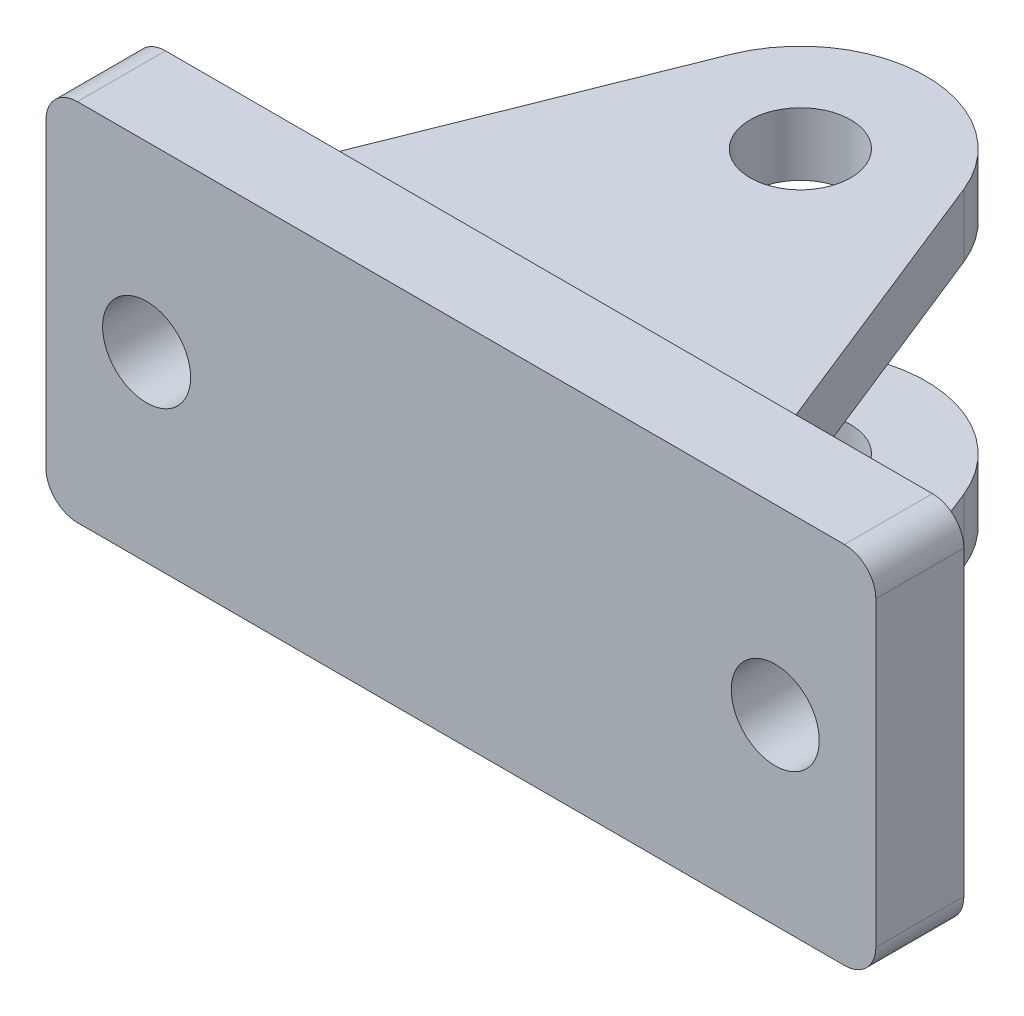
ISO-10303-21;
HEADER;
FILE_DESCRIPTION(('STEP AP214'),'2;1');
FILE_NAME('part.step','',(''),(''),'','','');
FILE_SCHEMA(('AUTOMOTIVE_DESIGN { 1 0 10303 214 1 1 1 1 }'));
ENDSEC;
DATA;
#1=APPLICATION_CONTEXT('core data for automotive mechanical design processes');
#2=APPLICATION_PROTOCOL_DEFINITION('international standard','automotive_design',2000,#1);
#3=PRODUCT_CONTEXT('',#1,'mechanical');
#4=PRODUCT('Part','Part','',(#3));
#5=PRODUCT_RELATED_PRODUCT_CATEGORY('part','',(#4));
#6=PRODUCT_DEFINITION_FORMATION('','',#4);
#7=PRODUCT_DEFINITION_CONTEXT('part definition',#1,'design');
#8=PRODUCT_DEFINITION('design','',#6,#7);
#9=PRODUCT_DEFINITION_SHAPE('','',#8);
#10=(LENGTH_UNIT() NAMED_UNIT(*) SI_UNIT(.MILLI.,.METRE.));
#11=(NAMED_UNIT(*) PLANE_ANGLE_UNIT() SI_UNIT($,.RADIAN.));
#12=(NAMED_UNIT(*) SI_UNIT($,.STERADIAN.) SOLID_ANGLE_UNIT());
#13=UNCERTAINTY_MEASURE_WITH_UNIT(LENGTH_MEASURE(1.E-05),#10,'distance_accuracy_value','');
#14=(GEOMETRIC_REPRESENTATION_CONTEXT(3) GLOBAL_UNCERTAINTY_ASSIGNED_CONTEXT((#13)) GLOBAL_UNIT_ASSIGNED_CONTEXT((#10,
#11,#12)) REPRESENTATION_CONTEXT('',''));
#15=CARTESIAN_POINT('',(0.,0.,0.));
#16=DIRECTION('',(0.,0.,1.));
#17=DIRECTION('',(1.,0.,0.));
#18=AXIS2_PLACEMENT_3D('',#15,#16,#17);
#19=CARTESIAN_POINT('',(-61.,24.,0.));
#20=DIRECTION('',(0.,0.,-1.));
#21=DIRECTION('',(-1.,0.,0.));
#22=AXIS2_PLACEMENT_3D('',#19,#20,#21);
#23=PLANE('',#22);
#24=DIRECTION('',(1.,0.,0.));
#25=VECTOR('',#24,1.);
#26=CARTESIAN_POINT('',(-37.5,-26.,0.));
#27=LINE('',#26,#25);
#28=CARTESIAN_POINT('',(-37.5,-26.,0.));
#29=VERTEX_POINT('',#28);
#30=CARTESIAN_POINT('',(37.5,-26.,0.));
#31=VERTEX_POINT('',#30);
#32=EDGE_CURVE('E176',#29,#31,#27,.T.);
#33=ORIENTED_EDGE('',*,*,#32,.T.);
#34=DIRECTION('',(0.,1.,0.));
#35=VECTOR('',#34,1.);
#36=CARTESIAN_POINT('',(37.5,-26.,0.));
#37=LINE('',#36,#35);
#38=CARTESIAN_POINT('',(37.5,-16.,0.));
#39=VERTEX_POINT('',#38);
#40=EDGE_CURVE('E163',#31,#39,#37,.T.);
#41=ORIENTED_EDGE('',*,*,#40,.T.);
#42=DIRECTION('',(1.,0.,0.));
#43=VECTOR('',#42,1.);
#44=CARTESIAN_POINT('',(-37.5,-16.,0.));
#45=LINE('',#44,#43);
#46=CARTESIAN_POINT('',(-37.5,-16.,0.));
#47=VERTEX_POINT('',#46);
#48=EDGE_CURVE('E189',#47,#39,#45,.T.);
#49=ORIENTED_EDGE('',*,*,#48,.F.);
#50=DIRECTION('',(0.,1.,0.));
#51=VECTOR('',#50,1.);
#52=CARTESIAN_POINT('',(-37.5,-26.,0.));
#53=LINE('',#52,#51);
#54=EDGE_CURVE('E191',#29,#47,#53,.T.);
#55=ORIENTED_EDGE('',*,*,#54,.F.);
#56=EDGE_LOOP('',(#33,#41,#49,#55));
#57=FACE_BOUND('',#56,.T.);
#58=CARTESIAN_POINT('',(-50.,0.,0.));
#59=DIRECTION('',(0.,0.,1.));
#60=DIRECTION('',(1.,0.,0.));
#61=AXIS2_PLACEMENT_3D('',#58,#59,#60);
#62=CIRCLE('',#61,7.);
#63=CARTESIAN_POINT('',(-43.,0.,0.));
#64=VERTEX_POINT('',#63);
#65=EDGE_CURVE('E235',#64,#64,#62,.T.);
#66=ORIENTED_EDGE('',*,*,#65,.T.);
#67=EDGE_LOOP('',(#66));
#68=FACE_BOUND('',#67,.T.);
#69=CARTESIAN_POINT('',(-61.,24.,0.));
#70=DIRECTION('',(0.,0.,1.));
#71=DIRECTION('',(-1.,0.,0.));
#72=AXIS2_PLACEMENT_3D('',#69,#70,#71);
#73=CIRCLE('',#72,5.);
#74=CARTESIAN_POINT('',(-61.,29.,0.));
#75=VERTEX_POINT('',#74);
#76=CARTESIAN_POINT('',(-66.,24.,0.));
#77=VERTEX_POINT('',#76);
#78=EDGE_CURVE('E236',#75,#77,#73,.T.);
#79=ORIENTED_EDGE('',*,*,#78,.F.);
#80=DIRECTION('',(-1.,0.,0.));
#81=VECTOR('',#80,1.);
#82=CARTESIAN_POINT('',(-61.,29.,0.));
#83=LINE('',#82,#81);
#84=CARTESIAN_POINT('',(61.,29.,0.));
#85=VERTEX_POINT('',#84);
#86=EDGE_CURVE('E241',#85,#75,#83,.T.);
#87=ORIENTED_EDGE('',*,*,#86,.F.);
#88=CARTESIAN_POINT('',(61.,24.,0.));
#89=DIRECTION('',(0.,0.,1.));
#90=DIRECTION('',(-1.,0.,0.));
#91=AXIS2_PLACEMENT_3D('',#88,#89,#90);
#92=CIRCLE('',#91,5.);
#93=CARTESIAN_POINT('',(66.,24.,0.));
#94=VERTEX_POINT('',#93);
#95=EDGE_CURVE('E275',#94,#85,#92,.T.);
#96=ORIENTED_EDGE('',*,*,#95,.F.);
#97=DIRECTION('',(0.,1.,0.));
#98=VECTOR('',#97,1.);
#99=CARTESIAN_POINT('',(66.,24.,0.));
#100=LINE('',#99,#98);
#101=CARTESIAN_POINT('',(66.,-24.,0.));
#102=VERTEX_POINT('',#101);
#103=EDGE_CURVE('E269',#102,#94,#100,.T.);
#104=ORIENTED_EDGE('',*,*,#103,.F.);
#105=CARTESIAN_POINT('',(61.,-24.,0.));
#106=DIRECTION('',(0.,0.,1.));
#107=DIRECTION('',(1.,0.,0.));
#108=AXIS2_PLACEMENT_3D('',#105,#106,#107);
#109=CIRCLE('',#108,5.);
#110=CARTESIAN_POINT('',(61.,-29.,0.));
#111=VERTEX_POINT('',#110);
#112=EDGE_CURVE('E268',#111,#102,#109,.T.);
#113=ORIENTED_EDGE('',*,*,#112,.F.);
#114=DIRECTION('',(1.,0.,0.));
#115=VECTOR('',#114,1.);
#116=CARTESIAN_POINT('',(-61.,-29.,0.));
#117=LINE('',#116,#115);
#118=CARTESIAN_POINT('',(-61.,-29.,0.));
#119=VERTEX_POINT('',#118);
#120=EDGE_CURVE('E266',#119,#111,#117,.T.);
#121=ORIENTED_EDGE('',*,*,#120,.F.);
#122=CARTESIAN_POINT('',(-61.,-24.,0.));
#123=DIRECTION('',(0.,0.,1.));
#124=DIRECTION('',(-1.,0.,0.));
#125=AXIS2_PLACEMENT_3D('',#122,#123,#124);
#126=CIRCLE('',#125,5.);
#127=CARTESIAN_POINT('',(-66.,-24.,0.));
#128=VERTEX_POINT('',#127);
#129=EDGE_CURVE('E262',#128,#119,#126,.T.);
#130=ORIENTED_EDGE('',*,*,#129,.F.);
#131=DIRECTION('',(0.,-1.,0.));
#132=VECTOR('',#131,1.);
#133=CARTESIAN_POINT('',(-66.,24.,0.));
#134=LINE('',#133,#132);
#135=EDGE_CURVE('E265',#77,#128,#134,.T.);
#136=ORIENTED_EDGE('',*,*,#135,.F.);
#137=EDGE_LOOP('',(#79,#87,#96,#104,#113,#121,#130,#136));
#138=FACE_BOUND('',#137,.T.);
#139=CARTESIAN_POINT('',(50.,0.,0.));
#140=DIRECTION('',(0.,0.,1.));
#141=DIRECTION('',(-1.,0.,0.));
#142=AXIS2_PLACEMENT_3D('',#139,#140,#141);
#143=CIRCLE('',#142,7.);
#144=CARTESIAN_POINT('',(43.,0.,0.));
#145=VERTEX_POINT('',#144);
#146=EDGE_CURVE('E227',#145,#145,#143,.T.);
#147=ORIENTED_EDGE('',*,*,#146,.T.);
#148=EDGE_LOOP('',(#147));
#149=FACE_BOUND('',#148,.T.);
#150=DIRECTION('',(1.,0.,0.));
#151=VECTOR('',#150,1.);
#152=CARTESIAN_POINT('',(-37.5,26.,0.));
#153=LINE('',#152,#151);
#154=CARTESIAN_POINT('',(-37.5,26.,0.));
#155=VERTEX_POINT('',#154);
#156=CARTESIAN_POINT('',(37.5,26.,0.));
#157=VERTEX_POINT('',#156);
#158=EDGE_CURVE('E206',#155,#157,#153,.T.);
#159=ORIENTED_EDGE('',*,*,#158,.F.);
#160=DIRECTION('',(0.,-1.,0.));
#161=VECTOR('',#160,1.);
#162=CARTESIAN_POINT('',(-37.5,26.,0.));
#163=LINE('',#162,#161);
#164=CARTESIAN_POINT('',(-37.5,16.,0.));
#165=VERTEX_POINT('',#164);
#166=EDGE_CURVE('E225',#155,#165,#163,.T.);
#167=ORIENTED_EDGE('',*,*,#166,.T.);
#168=DIRECTION('',(1.,0.,0.));
#169=VECTOR('',#168,1.);
#170=CARTESIAN_POINT('',(-37.5,16.,0.));
#171=LINE('',#170,#169);
#172=CARTESIAN_POINT('',(37.5,16.,0.));
#173=VERTEX_POINT('',#172);
#174=EDGE_CURVE('E212',#165,#173,#171,.T.);
#175=ORIENTED_EDGE('',*,*,#174,.T.);
#176=DIRECTION('',(0.,-1.,0.));
#177=VECTOR('',#176,1.);
#178=CARTESIAN_POINT('',(37.5,26.,0.));
#179=LINE('',#178,#177);
#180=EDGE_CURVE('E219',#157,#173,#179,.T.);
#181=ORIENTED_EDGE('',*,*,#180,.F.);
#182=EDGE_LOOP('',(#159,#167,#175,#181));
#183=FACE_BOUND('',#182,.T.);
#184=ADVANCED_FACE('F39',(#57,#68,#138,#149,#183),#23,.T.);
#185=CARTESIAN_POINT('',(-61.,24.,14.));
#186=DIRECTION('',(0.,0.,-1.));
#187=DIRECTION('',(-1.,0.,0.));
#188=AXIS2_PLACEMENT_3D('',#185,#186,#187);
#189=PLANE('',#188);
#190=CARTESIAN_POINT('',(-61.,24.,14.));
#191=DIRECTION('',(0.,0.,1.));
#192=DIRECTION('',(-1.,0.,0.));
#193=AXIS2_PLACEMENT_3D('',#190,#191,#192);
#194=CIRCLE('',#193,5.);
#195=CARTESIAN_POINT('',(-61.,29.,14.));
#196=VERTEX_POINT('',#195);
#197=CARTESIAN_POINT('',(-66.,24.,14.));
#198=VERTEX_POINT('',#197);
#199=EDGE_CURVE('E243',#196,#198,#194,.T.);
#200=ORIENTED_EDGE('',*,*,#199,.T.);
#201=DIRECTION('',(0.,-1.,0.));
#202=VECTOR('',#201,1.);
#203=CARTESIAN_POINT('',(-66.,24.,14.));
#204=LINE('',#203,#202);
#205=CARTESIAN_POINT('',(-66.,-24.,14.));
#206=VERTEX_POINT('',#205);
#207=EDGE_CURVE('E245',#198,#206,#204,.T.);
#208=ORIENTED_EDGE('',*,*,#207,.T.);
#209=CARTESIAN_POINT('',(-61.,-24.,14.));
#210=DIRECTION('',(0.,0.,1.));
#211=DIRECTION('',(-1.,0.,0.));
#212=AXIS2_PLACEMENT_3D('',#209,#210,#211);
#213=CIRCLE('',#212,5.);
#214=CARTESIAN_POINT('',(-61.,-29.,14.));
#215=VERTEX_POINT('',#214);
#216=EDGE_CURVE('E250',#206,#215,#213,.T.);
#217=ORIENTED_EDGE('',*,*,#216,.T.);
#218=DIRECTION('',(1.,0.,0.));
#219=VECTOR('',#218,1.);
#220=CARTESIAN_POINT('',(-61.,-29.,14.));
#221=LINE('',#220,#219);
#222=CARTESIAN_POINT('',(61.,-29.,14.));
#223=VERTEX_POINT('',#222);
#224=EDGE_CURVE('E248',#215,#223,#221,.T.);
#225=ORIENTED_EDGE('',*,*,#224,.T.);
#226=CARTESIAN_POINT('',(61.,-24.,14.));
#227=DIRECTION('',(0.,0.,1.));
#228=DIRECTION('',(1.,0.,0.));
#229=AXIS2_PLACEMENT_3D('',#226,#227,#228);
#230=CIRCLE('',#229,5.);
#231=CARTESIAN_POINT('',(66.,-24.,14.));
#232=VERTEX_POINT('',#231);
#233=EDGE_CURVE('E253',#223,#232,#230,.T.);
#234=ORIENTED_EDGE('',*,*,#233,.T.);
#235=DIRECTION('',(0.,1.,0.));
#236=VECTOR('',#235,1.);
#237=CARTESIAN_POINT('',(66.,24.,14.));
#238=LINE('',#237,#236);
#239=CARTESIAN_POINT('',(66.,24.,14.));
#240=VERTEX_POINT('',#239);
#241=EDGE_CURVE('E251',#232,#240,#238,.T.);
#242=ORIENTED_EDGE('',*,*,#241,.T.);
#243=CARTESIAN_POINT('',(61.,24.,14.));
#244=DIRECTION('',(0.,0.,1.));
#245=DIRECTION('',(-1.,0.,0.));
#246=AXIS2_PLACEMENT_3D('',#243,#244,#245);
#247=CIRCLE('',#246,5.);
#248=CARTESIAN_POINT('',(61.,29.,14.));
#249=VERTEX_POINT('',#248);
#250=EDGE_CURVE('E254',#240,#249,#247,.T.);
#251=ORIENTED_EDGE('',*,*,#250,.T.);
#252=DIRECTION('',(-1.,0.,0.));
#253=VECTOR('',#252,1.);
#254=CARTESIAN_POINT('',(-61.,29.,14.));
#255=LINE('',#254,#253);
#256=EDGE_CURVE('E260',#249,#196,#255,.T.);
#257=ORIENTED_EDGE('',*,*,#256,.T.);
#258=EDGE_LOOP('',(#200,#208,#217,#225,#234,#242,#251,#257));
#259=FACE_BOUND('',#258,.T.);
#260=CARTESIAN_POINT('',(-50.,0.,14.));
#261=DIRECTION('',(0.,0.,1.));
#262=DIRECTION('',(1.,0.,0.));
#263=AXIS2_PLACEMENT_3D('',#260,#261,#262);
#264=CIRCLE('',#263,7.);
#265=CARTESIAN_POINT('',(-43.,0.,14.));
#266=VERTEX_POINT('',#265);
#267=EDGE_CURVE('E234',#266,#266,#264,.T.);
#268=ORIENTED_EDGE('',*,*,#267,.F.);
#269=EDGE_LOOP('',(#268));
#270=FACE_BOUND('',#269,.T.);
#271=CARTESIAN_POINT('',(50.,0.,14.));
#272=DIRECTION('',(0.,0.,1.));
#273=DIRECTION('',(-1.,0.,0.));
#274=AXIS2_PLACEMENT_3D('',#271,#272,#273);
#275=CIRCLE('',#274,7.);
#276=CARTESIAN_POINT('',(43.,0.,14.));
#277=VERTEX_POINT('',#276);
#278=EDGE_CURVE('E230',#277,#277,#275,.T.);
#279=ORIENTED_EDGE('',*,*,#278,.F.);
#280=EDGE_LOOP('',(#279));
#281=FACE_BOUND('',#280,.T.);
#282=ADVANCED_FACE('F312',(#259,#270,#281),#189,.F.);
#283=CARTESIAN_POINT('',(-61.,24.,14.));
#284=DIRECTION('',(0.,0.,-1.));
#285=DIRECTION('',(-1.,0.,0.));
#286=AXIS2_PLACEMENT_3D('',#283,#284,#285);
#287=CYLINDRICAL_SURFACE('',#286,5.);
#288=ORIENTED_EDGE('',*,*,#78,.T.);
#289=DIRECTION('',(0.,0.,-1.));
#290=VECTOR('',#289,1.);
#291=CARTESIAN_POINT('',(-66.,24.,14.));
#292=LINE('',#291,#290);
#293=EDGE_CURVE('E11',#198,#77,#292,.T.);
#294=ORIENTED_EDGE('',*,*,#293,.F.);
#295=ORIENTED_EDGE('',*,*,#199,.F.);
#296=DIRECTION('',(0.,0.,-1.));
#297=VECTOR('',#296,1.);
#298=CARTESIAN_POINT('',(-61.,29.,14.));
#299=LINE('',#298,#297);
#300=EDGE_CURVE('E259',#196,#75,#299,.T.);
#301=ORIENTED_EDGE('',*,*,#300,.T.);
#302=EDGE_LOOP('',(#288,#294,#295,#301));
#303=FACE_BOUND('',#302,.T.);
#304=ADVANCED_FACE('F41',(#303),#287,.T.);
#305=CARTESIAN_POINT('',(-66.,24.,14.));
#306=DIRECTION('',(1.,0.,0.));
#307=DIRECTION('',(0.,0.,-1.));
#308=AXIS2_PLACEMENT_3D('',#305,#306,#307);
#309=PLANE('',#308);
#310=ORIENTED_EDGE('',*,*,#135,.T.);
#311=DIRECTION('',(0.,0.,-1.));
#312=VECTOR('',#311,1.);
#313=CARTESIAN_POINT('',(-66.,-24.,14.));
#314=LINE('',#313,#312);
#315=EDGE_CURVE('E50',#206,#128,#314,.T.);
#316=ORIENTED_EDGE('',*,*,#315,.F.);
#317=ORIENTED_EDGE('',*,*,#207,.F.);
#318=ORIENTED_EDGE('',*,*,#293,.T.);
#319=EDGE_LOOP('',(#310,#316,#317,#318));
#320=FACE_BOUND('',#319,.T.);
#321=ADVANCED_FACE('F319',(#320),#309,.F.);
#322=CARTESIAN_POINT('',(-61.,-24.,14.));
#323=DIRECTION('',(0.,0.,-1.));
#324=DIRECTION('',(-1.,0.,0.));
#325=AXIS2_PLACEMENT_3D('',#322,#323,#324);
#326=CYLINDRICAL_SURFACE('',#325,5.);
#327=ORIENTED_EDGE('',*,*,#129,.T.);
#328=DIRECTION('',(0.,0.,-1.));
#329=VECTOR('',#328,1.);
#330=CARTESIAN_POINT('',(-61.,-29.,14.));
#331=LINE('',#330,#329);
#332=EDGE_CURVE('E288',#215,#119,#331,.T.);
#333=ORIENTED_EDGE('',*,*,#332,.F.);
#334=ORIENTED_EDGE('',*,*,#216,.F.);
#335=ORIENTED_EDGE('',*,*,#315,.T.);
#336=EDGE_LOOP('',(#327,#333,#334,#335));
#337=FACE_BOUND('',#336,.T.);
#338=ADVANCED_FACE('F298',(#337),#326,.T.);
#339=CARTESIAN_POINT('',(-61.,-29.,14.));
#340=DIRECTION('',(0.,1.,0.));
#341=DIRECTION('',(0.,0.,1.));
#342=AXIS2_PLACEMENT_3D('',#339,#340,#341);
#343=PLANE('',#342);
#344=ORIENTED_EDGE('',*,*,#120,.T.);
#345=DIRECTION('',(0.,0.,-1.));
#346=VECTOR('',#345,1.);
#347=CARTESIAN_POINT('',(61.,-29.,14.));
#348=LINE('',#347,#346);
#349=EDGE_CURVE('E286',#223,#111,#348,.T.);
#350=ORIENTED_EDGE('',*,*,#349,.F.);
#351=ORIENTED_EDGE('',*,*,#224,.F.);
#352=ORIENTED_EDGE('',*,*,#332,.T.);
#353=EDGE_LOOP('',(#344,#350,#351,#352));
#354=FACE_BOUND('',#353,.T.);
#355=ADVANCED_FACE('F307',(#354),#343,.F.);
#356=CARTESIAN_POINT('',(61.,-24.,14.));
#357=DIRECTION('',(0.,0.,-1.));
#358=DIRECTION('',(-1.,0.,0.));
#359=AXIS2_PLACEMENT_3D('',#356,#357,#358);
#360=CYLINDRICAL_SURFACE('',#359,5.);
#361=ORIENTED_EDGE('',*,*,#112,.T.);
#362=DIRECTION('',(0.,0.,-1.));
#363=VECTOR('',#362,1.);
#364=CARTESIAN_POINT('',(66.,-24.,14.));
#365=LINE('',#364,#363);
#366=EDGE_CURVE('E282',#232,#102,#365,.T.);
#367=ORIENTED_EDGE('',*,*,#366,.F.);
#368=ORIENTED_EDGE('',*,*,#233,.F.);
#369=ORIENTED_EDGE('',*,*,#349,.T.);
#370=EDGE_LOOP('',(#361,#367,#368,#369));
#371=FACE_BOUND('',#370,.T.);
#372=ADVANCED_FACE('F313',(#371),#360,.T.);
#373=CARTESIAN_POINT('',(66.,24.,14.));
#374=DIRECTION('',(-1.,0.,0.));
#375=DIRECTION('',(0.,-1.,0.));
#376=AXIS2_PLACEMENT_3D('',#373,#374,#375);
#377=PLANE('',#376);
#378=ORIENTED_EDGE('',*,*,#103,.T.);
#379=DIRECTION('',(0.,0.,-1.));
#380=VECTOR('',#379,1.);
#381=CARTESIAN_POINT('',(66.,24.,14.));
#382=LINE('',#381,#380);
#383=EDGE_CURVE('E278',#240,#94,#382,.T.);
#384=ORIENTED_EDGE('',*,*,#383,.F.);
#385=ORIENTED_EDGE('',*,*,#241,.F.);
#386=ORIENTED_EDGE('',*,*,#366,.T.);
#387=EDGE_LOOP('',(#378,#384,#385,#386));
#388=FACE_BOUND('',#387,.T.);
#389=ADVANCED_FACE('F334',(#388),#377,.F.);
#390=CARTESIAN_POINT('',(61.,24.,14.));
#391=DIRECTION('',(0.,0.,-1.));
#392=DIRECTION('',(-1.,0.,0.));
#393=AXIS2_PLACEMENT_3D('',#390,#391,#392);
#394=CYLINDRICAL_SURFACE('',#393,5.);
#395=ORIENTED_EDGE('',*,*,#95,.T.);
#396=DIRECTION('',(0.,0.,-1.));
#397=VECTOR('',#396,1.);
#398=CARTESIAN_POINT('',(61.,29.,14.));
#399=LINE('',#398,#397);
#400=EDGE_CURVE('E280',#249,#85,#399,.T.);
#401=ORIENTED_EDGE('',*,*,#400,.F.);
#402=ORIENTED_EDGE('',*,*,#250,.F.);
#403=ORIENTED_EDGE('',*,*,#383,.T.);
#404=EDGE_LOOP('',(#395,#401,#402,#403));
#405=FACE_BOUND('',#404,.T.);
#406=ADVANCED_FACE('F332',(#405),#394,.T.);
#407=CARTESIAN_POINT('',(-61.,29.,14.));
#408=DIRECTION('',(0.,-1.,0.));
#409=DIRECTION('',(0.,0.,-1.));
#410=AXIS2_PLACEMENT_3D('',#407,#408,#409);
#411=PLANE('',#410);
#412=ORIENTED_EDGE('',*,*,#86,.T.);
#413=ORIENTED_EDGE('',*,*,#300,.F.);
#414=ORIENTED_EDGE('',*,*,#256,.F.);
#415=ORIENTED_EDGE('',*,*,#400,.T.);
#416=EDGE_LOOP('',(#412,#413,#414,#415));
#417=FACE_BOUND('',#416,.T.);
#418=ADVANCED_FACE('F326',(#417),#411,.F.);
#419=CARTESIAN_POINT('',(-50.,0.,14.));
#420=DIRECTION('',(0.,0.,-1.));
#421=DIRECTION('',(-1.,0.,0.));
#422=AXIS2_PLACEMENT_3D('',#419,#420,#421);
#423=CYLINDRICAL_SURFACE('',#422,7.);
#424=ORIENTED_EDGE('',*,*,#267,.T.);
#425=EDGE_LOOP('',(#424));
#426=FACE_BOUND('',#425,.T.);
#427=ORIENTED_EDGE('',*,*,#65,.F.);
#428=EDGE_LOOP('',(#427));
#429=FACE_BOUND('',#428,.T.);
#430=ADVANCED_FACE('F351',(#426,#429),#423,.F.);
#431=CARTESIAN_POINT('',(50.,0.,14.));
#432=DIRECTION('',(0.,0.,-1.));
#433=DIRECTION('',(-1.,0.,0.));
#434=AXIS2_PLACEMENT_3D('',#431,#432,#433);
#435=CYLINDRICAL_SURFACE('',#434,7.);
#436=ORIENTED_EDGE('',*,*,#278,.T.);
#437=EDGE_LOOP('',(#436));
#438=FACE_BOUND('',#437,.T.);
#439=ORIENTED_EDGE('',*,*,#146,.F.);
#440=EDGE_LOOP('',(#439));
#441=FACE_BOUND('',#440,.T.);
#442=ADVANCED_FACE('F358',(#438,#441),#435,.F.);
#443=CARTESIAN_POINT('',(0.,26.,-40.));
#444=DIRECTION('',(0.,1.,0.));
#445=DIRECTION('',(0.,0.,1.));
#446=AXIS2_PLACEMENT_3D('',#443,#444,#445);
#447=PLANE('',#446);
#448=CARTESIAN_POINT('',(0.,26.,-40.));
#449=DIRECTION('',(0.,1.,0.));
#450=DIRECTION('',(0.,0.,1.));
#451=AXIS2_PLACEMENT_3D('',#448,#449,#450);
#452=CIRCLE('',#451,20.);
#453=CARTESIAN_POINT('',(18.5750206115008,26.,-47.414081823282));
#454=VERTEX_POINT('',#453);
#455=CARTESIAN_POINT('',(-18.5750206115008,26.,-47.414081823282));
#456=VERTEX_POINT('',#455);
#457=EDGE_CURVE('E199',#454,#456,#452,.T.);
#458=ORIENTED_EDGE('',*,*,#457,.T.);
#459=DIRECTION('',(-0.3707040911641,0.,0.92875103057504));
#460=VECTOR('',#459,1.);
#461=CARTESIAN_POINT('',(-37.5,26.,0.));
#462=LINE('',#461,#460);
#463=EDGE_CURVE('E201',#456,#155,#462,.T.);
#464=ORIENTED_EDGE('',*,*,#463,.T.);
#465=ORIENTED_EDGE('',*,*,#158,.T.);
#466=DIRECTION('',(-0.3707040911641,0.,-0.92875103057504));
#467=VECTOR('',#466,1.);
#468=CARTESIAN_POINT('',(37.5,26.,0.));
#469=LINE('',#468,#467);
#470=EDGE_CURVE('E64',#157,#454,#469,.T.);
#471=ORIENTED_EDGE('',*,*,#470,.T.);
#472=EDGE_LOOP('',(#458,#464,#465,#471));
#473=FACE_BOUND('',#472,.T.);
#474=CARTESIAN_POINT('',(0.,26.,-40.));
#475=DIRECTION('',(0.,1.,0.));
#476=DIRECTION('',(0.,0.,1.));
#477=AXIS2_PLACEMENT_3D('',#474,#475,#476);
#478=CIRCLE('',#477,8.);
#479=CARTESIAN_POINT('',(0.,26.,-32.));
#480=VERTEX_POINT('',#479);
#481=EDGE_CURVE('E193',#480,#480,#478,.T.);
#482=ORIENTED_EDGE('',*,*,#481,.F.);
#483=EDGE_LOOP('',(#482));
#484=FACE_BOUND('',#483,.T.);
#485=ADVANCED_FACE('F365',(#473,#484),#447,.T.);
#486=CARTESIAN_POINT('',(0.,16.,-40.));
#487=DIRECTION('',(0.,1.,0.));
#488=DIRECTION('',(0.,0.,1.));
#489=AXIS2_PLACEMENT_3D('',#486,#487,#488);
#490=PLANE('',#489);
#491=CARTESIAN_POINT('',(0.,16.,-40.));
#492=DIRECTION('',(0.,1.,0.));
#493=DIRECTION('',(0.,0.,1.));
#494=AXIS2_PLACEMENT_3D('',#491,#492,#493);
#495=CIRCLE('',#494,20.);
#496=CARTESIAN_POINT('',(18.5750206115008,16.,-47.414081823282));
#497=VERTEX_POINT('',#496);
#498=CARTESIAN_POINT('',(-18.5750206115008,16.,-47.414081823282));
#499=VERTEX_POINT('',#498);
#500=EDGE_CURVE('E197',#497,#499,#495,.T.);
#501=ORIENTED_EDGE('',*,*,#500,.F.);
#502=DIRECTION('',(-0.3707040911641,0.,-0.92875103057504));
#503=VECTOR('',#502,1.);
#504=CARTESIAN_POINT('',(37.5,16.,0.));
#505=LINE('',#504,#503);
#506=EDGE_CURVE('E204',#173,#497,#505,.T.);
#507=ORIENTED_EDGE('',*,*,#506,.F.);
#508=ORIENTED_EDGE('',*,*,#174,.F.);
#509=DIRECTION('',(-0.3707040911641,0.,0.92875103057504));
#510=VECTOR('',#509,1.);
#511=CARTESIAN_POINT('',(-37.5,16.,0.));
#512=LINE('',#511,#510);
#513=EDGE_CURVE('E215',#499,#165,#512,.T.);
#514=ORIENTED_EDGE('',*,*,#513,.F.);
#515=EDGE_LOOP('',(#501,#507,#508,#514));
#516=FACE_BOUND('',#515,.T.);
#517=CARTESIAN_POINT('',(0.,16.,-40.));
#518=DIRECTION('',(0.,1.,0.));
#519=DIRECTION('',(0.,0.,1.));
#520=AXIS2_PLACEMENT_3D('',#517,#518,#519);
#521=CIRCLE('',#520,8.);
#522=CARTESIAN_POINT('',(0.,16.,-32.));
#523=VERTEX_POINT('',#522);
#524=EDGE_CURVE('E162',#523,#523,#521,.T.);
#525=ORIENTED_EDGE('',*,*,#524,.T.);
#526=EDGE_LOOP('',(#525));
#527=FACE_BOUND('',#526,.T.);
#528=ADVANCED_FACE('F373',(#516,#527),#490,.F.);
#529=CARTESIAN_POINT('',(0.,26.,-40.));
#530=DIRECTION('',(0.,-1.,0.));
#531=DIRECTION('',(0.,0.,-1.));
#532=AXIS2_PLACEMENT_3D('',#529,#530,#531);
#533=CYLINDRICAL_SURFACE('',#532,20.);
#534=ORIENTED_EDGE('',*,*,#500,.T.);
#535=DIRECTION('',(0.,-1.,0.));
#536=VECTOR('',#535,1.);
#537=CARTESIAN_POINT('',(-18.5750206115008,26.,-47.414081823282));
#538=LINE('',#537,#536);
#539=EDGE_CURVE('E223',#456,#499,#538,.T.);
#540=ORIENTED_EDGE('',*,*,#539,.F.);
#541=ORIENTED_EDGE('',*,*,#457,.F.);
#542=DIRECTION('',(0.,-1.,0.));
#543=VECTOR('',#542,1.);
#544=CARTESIAN_POINT('',(18.5750206115008,26.,-47.414081823282));
#545=LINE('',#544,#543);
#546=EDGE_CURVE('E207',#454,#497,#545,.T.);
#547=ORIENTED_EDGE('',*,*,#546,.T.);
#548=EDGE_LOOP('',(#534,#540,#541,#547));
#549=FACE_BOUND('',#548,.T.);
#550=ADVANCED_FACE('F369',(#549),#533,.T.);
#551=CARTESIAN_POINT('',(-37.5,26.,0.));
#552=DIRECTION('',(0.92875103057504,0.,0.3707040911641));
#553=DIRECTION('',(0.3707040911641,0.,-0.92875103057504));
#554=AXIS2_PLACEMENT_3D('',#551,#552,#553);
#555=PLANE('',#554);
#556=ORIENTED_EDGE('',*,*,#513,.T.);
#557=ORIENTED_EDGE('',*,*,#166,.F.);
#558=ORIENTED_EDGE('',*,*,#463,.F.);
#559=ORIENTED_EDGE('',*,*,#539,.T.);
#560=EDGE_LOOP('',(#556,#557,#558,#559));
#561=FACE_BOUND('',#560,.T.);
#562=ADVANCED_FACE('F375',(#561),#555,.F.);
#563=CARTESIAN_POINT('',(37.5,26.,0.));
#564=DIRECTION('',(-0.92875103057504,0.,0.3707040911641));
#565=DIRECTION('',(0.3707040911641,0.,0.92875103057504));
#566=AXIS2_PLACEMENT_3D('',#563,#564,#565);
#567=PLANE('',#566);
#568=ORIENTED_EDGE('',*,*,#506,.T.);
#569=ORIENTED_EDGE('',*,*,#546,.F.);
#570=ORIENTED_EDGE('',*,*,#470,.F.);
#571=ORIENTED_EDGE('',*,*,#180,.T.);
#572=EDGE_LOOP('',(#568,#569,#570,#571));
#573=FACE_BOUND('',#572,.T.);
#574=ADVANCED_FACE('F380',(#573),#567,.F.);
#575=CARTESIAN_POINT('',(0.,26.,-40.));
#576=DIRECTION('',(0.,-1.,0.));
#577=DIRECTION('',(0.,0.,-1.));
#578=AXIS2_PLACEMENT_3D('',#575,#576,#577);
#579=CYLINDRICAL_SURFACE('',#578,8.);
#580=ORIENTED_EDGE('',*,*,#481,.T.);
#581=EDGE_LOOP('',(#580));
#582=FACE_BOUND('',#581,.T.);
#583=ORIENTED_EDGE('',*,*,#524,.F.);
#584=EDGE_LOOP('',(#583));
#585=FACE_BOUND('',#584,.T.);
#586=ADVANCED_FACE('F381',(#582,#585),#579,.F.);
#587=CARTESIAN_POINT('',(0.,-26.,-40.));
#588=DIRECTION('',(0.,1.,0.));
#589=DIRECTION('',(0.,0.,1.));
#590=AXIS2_PLACEMENT_3D('',#587,#588,#589);
#591=CYLINDRICAL_SURFACE('',#590,20.);
#592=CARTESIAN_POINT('',(0.,-16.,-40.));
#593=DIRECTION('',(0.,1.,0.));
#594=DIRECTION('',(0.,0.,1.));
#595=AXIS2_PLACEMENT_3D('',#592,#593,#594);
#596=CIRCLE('',#595,20.);
#597=CARTESIAN_POINT('',(18.5750206115008,-16.,-47.414081823282));
#598=VERTEX_POINT('',#597);
#599=CARTESIAN_POINT('',(-18.5750206115008,-16.,-47.414081823282));
#600=VERTEX_POINT('',#599);
#601=EDGE_CURVE('E157',#598,#600,#596,.T.);
#602=ORIENTED_EDGE('',*,*,#601,.F.);
#603=DIRECTION('',(0.,1.,0.));
#604=VECTOR('',#603,1.);
#605=CARTESIAN_POINT('',(18.5750206115008,-26.,-47.414081823282));
#606=LINE('',#605,#604);
#607=CARTESIAN_POINT('',(18.5750206115008,-26.,-47.414081823282));
#608=VERTEX_POINT('',#607);
#609=EDGE_CURVE('E152',#608,#598,#606,.T.);
#610=ORIENTED_EDGE('',*,*,#609,.F.);
#611=CARTESIAN_POINT('',(0.,-26.,-40.));
#612=DIRECTION('',(0.,1.,0.));
#613=DIRECTION('',(0.,0.,1.));
#614=AXIS2_PLACEMENT_3D('',#611,#612,#613);
#615=CIRCLE('',#614,20.);
#616=CARTESIAN_POINT('',(-18.5750206115008,-26.,-47.414081823282));
#617=VERTEX_POINT('',#616);
#618=EDGE_CURVE('E160',#608,#617,#615,.T.);
#619=ORIENTED_EDGE('',*,*,#618,.T.);
#620=DIRECTION('',(0.,1.,0.));
#621=VECTOR('',#620,1.);
#622=CARTESIAN_POINT('',(-18.5750206115008,-26.,-47.414081823282));
#623=LINE('',#622,#621);
#624=EDGE_CURVE('E185',#617,#600,#623,.T.);
#625=ORIENTED_EDGE('',*,*,#624,.T.);
#626=EDGE_LOOP('',(#602,#610,#619,#625));
#627=FACE_BOUND('',#626,.T.);
#628=ADVANCED_FACE('F156',(#627),#591,.T.);
#629=CARTESIAN_POINT('',(37.5,-26.,0.));
#630=DIRECTION('',(0.92875103057504,0.,-0.3707040911641));
#631=DIRECTION('',(-0.3707040911641,0.,-0.92875103057504));
#632=AXIS2_PLACEMENT_3D('',#629,#630,#631);
#633=PLANE('',#632);
#634=DIRECTION('',(-0.3707040911641,0.,-0.92875103057504));
#635=VECTOR('',#634,1.);
#636=CARTESIAN_POINT('',(37.5,-16.,0.));
#637=LINE('',#636,#635);
#638=EDGE_CURVE('E184',#39,#598,#637,.T.);
#639=ORIENTED_EDGE('',*,*,#638,.F.);
#640=ORIENTED_EDGE('',*,*,#40,.F.);
#641=DIRECTION('',(-0.3707040911641,0.,-0.92875103057504));
#642=VECTOR('',#641,1.);
#643=CARTESIAN_POINT('',(37.5,-26.,0.));
#644=LINE('',#643,#642);
#645=EDGE_CURVE('E166',#31,#608,#644,.T.);
#646=ORIENTED_EDGE('',*,*,#645,.T.);
#647=ORIENTED_EDGE('',*,*,#609,.T.);
#648=EDGE_LOOP('',(#639,#640,#646,#647));
#649=FACE_BOUND('',#648,.T.);
#650=ADVANCED_FACE('F175',(#649),#633,.T.);
#651=CARTESIAN_POINT('',(-37.5,-26.,0.));
#652=DIRECTION('',(-0.92875103057504,0.,-0.3707040911641));
#653=DIRECTION('',(-0.3707040911641,0.,0.92875103057504));
#654=AXIS2_PLACEMENT_3D('',#651,#652,#653);
#655=PLANE('',#654);
#656=DIRECTION('',(-0.3707040911641,0.,0.92875103057504));
#657=VECTOR('',#656,1.);
#658=CARTESIAN_POINT('',(-37.5,-16.,0.));
#659=LINE('',#658,#657);
#660=EDGE_CURVE('E53',#600,#47,#659,.T.);
#661=ORIENTED_EDGE('',*,*,#660,.F.);
#662=ORIENTED_EDGE('',*,*,#624,.F.);
#663=DIRECTION('',(-0.3707040911641,0.,0.92875103057504));
#664=VECTOR('',#663,1.);
#665=CARTESIAN_POINT('',(-37.5,-26.,0.));
#666=LINE('',#665,#664);
#667=EDGE_CURVE('E174',#617,#29,#666,.T.);
#668=ORIENTED_EDGE('',*,*,#667,.T.);
#669=ORIENTED_EDGE('',*,*,#54,.T.);
#670=EDGE_LOOP('',(#661,#662,#668,#669));
#671=FACE_BOUND('',#670,.T.);
#672=ADVANCED_FACE('F392',(#671),#655,.T.);
#673=CARTESIAN_POINT('',(0.,-26.,-40.));
#674=DIRECTION('',(0.,-1.,0.));
#675=DIRECTION('',(0.,0.,1.));
#676=AXIS2_PLACEMENT_3D('',#673,#674,#675);
#677=PLANE('',#676);
#678=CARTESIAN_POINT('',(0.,-26.,-40.));
#679=DIRECTION('',(0.,1.,0.));
#680=DIRECTION('',(0.,0.,1.));
#681=AXIS2_PLACEMENT_3D('',#678,#679,#680);
#682=CIRCLE('',#681,8.);
#683=CARTESIAN_POINT('',(0.,-26.,-32.));
#684=VERTEX_POINT('',#683);
#685=EDGE_CURVE('E183',#684,#684,#682,.T.);
#686=ORIENTED_EDGE('',*,*,#685,.T.);
#687=EDGE_LOOP('',(#686));
#688=FACE_BOUND('',#687,.T.);
#689=ORIENTED_EDGE('',*,*,#618,.F.);
#690=ORIENTED_EDGE('',*,*,#645,.F.);
#691=ORIENTED_EDGE('',*,*,#32,.F.);
#692=ORIENTED_EDGE('',*,*,#667,.F.);
#693=EDGE_LOOP('',(#689,#690,#691,#692));
#694=FACE_BOUND('',#693,.T.);
#695=ADVANCED_FACE('F169',(#688,#694),#677,.T.);
#696=CARTESIAN_POINT('',(0.,-16.,-40.));
#697=DIRECTION('',(0.,-1.,0.));
#698=DIRECTION('',(0.,0.,1.));
#699=AXIS2_PLACEMENT_3D('',#696,#697,#698);
#700=PLANE('',#699);
#701=CARTESIAN_POINT('',(0.,-16.,-40.));
#702=DIRECTION('',(0.,1.,0.));
#703=DIRECTION('',(0.,0.,1.));
#704=AXIS2_PLACEMENT_3D('',#701,#702,#703);
#705=CIRCLE('',#704,8.);
#706=CARTESIAN_POINT('',(0.,-16.,-32.));
#707=VERTEX_POINT('',#706);
#708=EDGE_CURVE('E413',#707,#707,#705,.T.);
#709=ORIENTED_EDGE('',*,*,#708,.F.);
#710=EDGE_LOOP('',(#709));
#711=FACE_BOUND('',#710,.T.);
#712=ORIENTED_EDGE('',*,*,#601,.T.);
#713=ORIENTED_EDGE('',*,*,#660,.T.);
#714=ORIENTED_EDGE('',*,*,#48,.T.);
#715=ORIENTED_EDGE('',*,*,#638,.T.);
#716=EDGE_LOOP('',(#712,#713,#714,#715));
#717=FACE_BOUND('',#716,.T.);
#718=ADVANCED_FACE('F400',(#711,#717),#700,.F.);
#719=CARTESIAN_POINT('',(0.,-26.,-40.));
#720=DIRECTION('',(0.,1.,0.));
#721=DIRECTION('',(0.,0.,1.));
#722=AXIS2_PLACEMENT_3D('',#719,#720,#721);
#723=CYLINDRICAL_SURFACE('',#722,8.);
#724=ORIENTED_EDGE('',*,*,#685,.F.);
#725=EDGE_LOOP('',(#724));
#726=FACE_BOUND('',#725,.T.);
#727=ORIENTED_EDGE('',*,*,#708,.T.);
#728=EDGE_LOOP('',(#727));
#729=FACE_BOUND('',#728,.T.);
#730=ADVANCED_FACE('F399',(#726,#729),#723,.F.);
#731=CLOSED_SHELL('',(#184,#282,#304,#321,#338,#355,#372,#389,#406,#418,#430,#442,#485,#528,
#550,#562,#574,#586,#628,#650,#672,#695,#718,#730));
#732=MANIFOLD_SOLID_BREP('B2',#731);
#733=ADVANCED_BREP_SHAPE_REPRESENTATION('',(#18,#732),#14);
#734=SHAPE_DEFINITION_REPRESENTATION(#9,#733);
ENDSEC;
END-ISO-10303-21;
